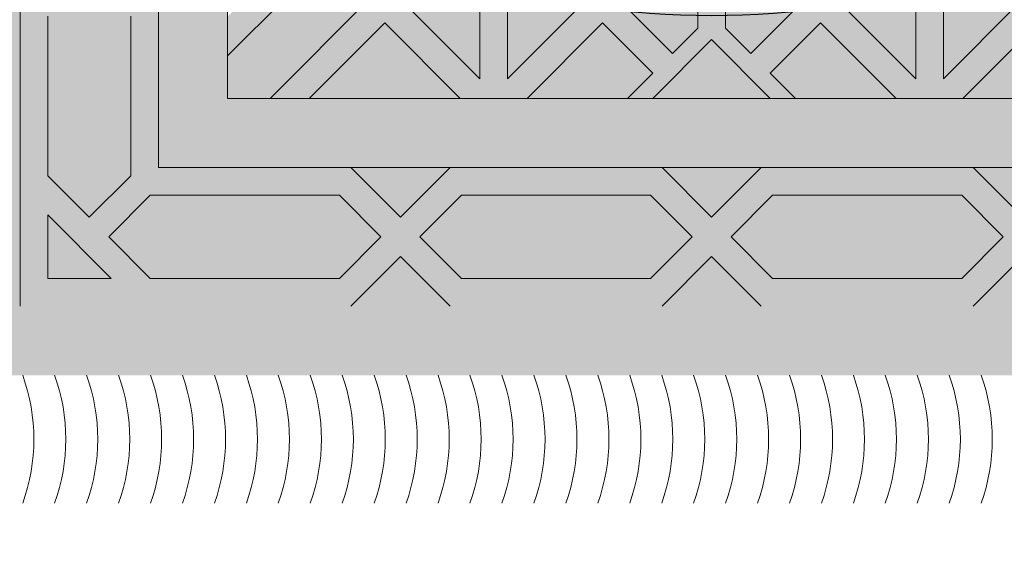
# Model space of a CAD drawing. Units: inches. Extents: x 844 to 2234, y 346 to 1084.
# Tile 69 of 93: x 1997.478 to 2006.557, y 687.628 to 692.525. Entities that reach past the tile are written whole.
import ezdxf

# ---------------------------------------------------------------- set-up
doc = ezdxf.new("R2010")
doc.units = ezdxf.units.IN
doc.header["$MEASUREMENT"] = 0
for name, color, linetype, lineweight in [('A-ANNO-DIMS', 2, 'Continuous', 18), ('furniture', 8, 'Continuous', 18), ('RA-AP-01$0$INT', 35, 'Continuous', 5)]:
    doc.layers.add(name, color=color, linetype=linetype, lineweight=lineweight)
doc.layers.add('RA-AP-01$0$FURN', color=3, linetype='Continuous')
doc.layers.add('RA-AP-01$0$WOOD', color=64, linetype='Continuous')
doc.styles.get("Standard").update_dxf_attribs({"font": 'arial.ttf'})
doc.dimstyles.get("Standard").update_dxf_attribs({"dimtxt": 6, "dimasz": 3, "dimexe": 0.18, "dimexo": 0.0625, "dimgap": 0.09, "dimtad": 0, "dimtih": 1, "dimtoh": 1, "dimdec": 1, "dimzin": 0, "dimdsep": 46, "dimlunit": 3, "dimtxsty": 'Standard', "dimblk": 'ARCHTICK', "dimcen": 0.09, "dimadec": 0, "dimazin": 0, "dimtfac": 1, "dimtdec": 1, "dimtofl": 0, "dimtmove": 0, "dimatfit": 3, "dimfxl": 1, "dimtolj": 1, "dimtzin": 0, "dimarcsym": 0})

# ---------------------------------------------------------------- blocks, each defined once
blk = doc.blocks.new('A$C18D01794')
at = {"layer": 'RA-AP-01$0$INT'}
h = blk.add_hatch(color=256, dxfattribs=at)
h.paths.add_polyline_path([(4.35521, -6.15671), (4.35521, -8.05671), (5.45521, -8.05671), (5.45521, -6.15671)])
h.paths.add_polyline_path([(4.40521, -8.00671), (4.40521, -6.20671), (5.40521, -6.20671), (5.40521, -8.00671)], flags=16)
h = blk.add_hatch(color=256, dxfattribs=at)
h.paths.add_polyline_path([(4.46935, -7.07085), (4.50521, -7.035), (4.50521, -7.10671)])
h.paths.add_polyline_path([(4.45521, -7.085), (4.47692, -7.10671), (4.43349, -7.10671)])
h.paths.add_polyline_path([(4.40521, -7.035), (4.44106, -7.07085), (4.40521, -7.10671)])
h.paths.add_polyline_path([(4.42521, -6.91146), (4.45521, -6.88146), (4.48521, -6.91146), (4.48521, -7.02671), (4.45521, -7.05671), (4.42521, -7.02671)])
h.paths.add_polyline_path([(4.50521, -6.83146), (4.50521, -6.90318), (4.46935, -6.86732)])
h.paths.add_polyline_path([(4.42521, -6.70793), (4.45521, -6.67793), (4.48521, -6.70793), (4.48521, -6.82318), (4.45521, -6.85318), (4.42521, -6.82318)])
h.paths.add_polyline_path([(4.42521, -6.50439), (4.45521, -6.47439), (4.48521, -6.50439), (4.48521, -6.61964), (4.45521, -6.64964), (4.42521, -6.61964)])
h.paths.add_polyline_path([(4.46935, -6.66378), (4.50521, -6.62793), (4.50521, -6.69964)])
h.paths.add_polyline_path([(4.40521, -6.62793), (4.44106, -6.66378), (4.40521, -6.69964)])
h.paths.add_polyline_path([(4.40521, -6.42439), (4.44106, -6.46025), (4.40521, -6.49611)])
h.paths.add_polyline_path([(4.46935, -6.46025), (4.50521, -6.42439), (4.50521, -6.49611)])
h.paths.add_polyline_path([(4.42521, -6.30085), (4.45521, -6.27085), (4.48521, -6.30085), (4.48521, -6.41611), (4.45521, -6.44611), (4.42521, -6.41611)])
h.paths.add_polyline_path([(4.42521, -6.22671), (4.47106, -6.22671), (4.42521, -6.27257)])
h.paths.add_polyline_path([(4.49935, -6.22671), (4.63606, -6.22671), (4.66606, -6.25671), (4.63606, -6.28671), (4.49935, -6.28671), (4.46935, -6.25671)])
h.paths.add_polyline_path([(4.68021, -6.27085), (4.71606, -6.30671), (4.64435, -6.30671)])
h.paths.add_polyline_path([(4.64435, -6.20671), (4.71606, -6.20671), (4.68021, -6.24257)])
h.paths.add_polyline_path([(4.72435, -6.22671), (4.86106, -6.22671), (4.89106, -6.25671), (4.86106, -6.28671), (4.72435, -6.28671), (4.69435, -6.25671)])
h.paths.add_polyline_path([(4.90521, -6.27085), (4.94106, -6.30671), (4.86935, -6.30671)])
h.paths.add_polyline_path([(4.86935, -6.20671), (4.94106, -6.20671), (4.90521, -6.24257)])
h.paths.add_polyline_path([(4.94935, -6.22671), (5.08606, -6.22671), (5.11606, -6.25671), (5.08606, -6.28671), (4.94935, -6.28671), (4.91935, -6.25671)])
h.paths.add_polyline_path([(5.13021, -6.27085), (5.16606, -6.30671), (5.09435, -6.30671)])
h.paths.add_polyline_path([(5.09435, -6.20671), (5.16606, -6.20671), (5.13021, -6.24257)])
h.paths.add_polyline_path([(5.17435, -6.22671), (5.31106, -6.22671), (5.34106, -6.25671), (5.31106, -6.28671), (5.17435, -6.28671), (5.14435, -6.25671)])
h.paths.add_polyline_path([(5.32521, -6.30085), (5.35521, -6.27085), (5.38521, -6.30085), (5.38521, -6.41611), (5.35521, -6.44611), (5.32521, -6.41611)])
h.paths.add_polyline_path([(5.33935, -6.22671), (5.38521, -6.22671), (5.38521, -6.27257)])
h.paths.add_polyline_path([(5.32521, -6.50439), (5.35521, -6.47439), (5.38521, -6.50439), (5.38521, -6.61964), (5.35521, -6.64964), (5.32521, -6.61964)])
h.paths.add_polyline_path([(5.30521, -6.42439), (5.34106, -6.46025), (5.30521, -6.49611)])
h.paths.add_polyline_path([(5.36935, -6.46025), (5.40521, -6.42439), (5.40521, -6.49611)])
h.paths.add_polyline_path([(5.40521, -6.62793), (5.40521, -6.69964), (5.36935, -6.66378)])
h.paths.add_polyline_path([(5.30521, -6.62793), (5.34106, -6.66378), (5.30521, -6.69964)])
h.paths.add_polyline_path([(5.32521, -6.70793), (5.35521, -6.67793), (5.38521, -6.70793), (5.38521, -6.82318), (5.35521, -6.85318), (5.32521, -6.82318)])
h.paths.add_polyline_path([(5.30521, -6.83146), (5.34106, -6.86732), (5.30521, -6.90318)])
h.paths.add_polyline_path([(5.32521, -6.91146), (5.35521, -6.88146), (5.38521, -6.91146), (5.38521, -7.02671), (5.35521, -7.05671), (5.32521, -7.02671)])
h.paths.add_polyline_path([(5.40458, -6.83209, 0.001218), (5.40521, -6.83231), (5.40521, -6.90318), (5.36935, -6.86732)])
h.paths.add_polyline_path([(5.36935, -7.07085), (5.40521, -7.035), (5.40521, -7.10671)])
h.paths.add_polyline_path([(5.35521, -7.085), (5.37692, -7.10671), (5.33349, -7.10671)])
h.paths.add_polyline_path([(5.30521, -7.035), (5.34106, -7.07085), (5.30521, -7.10671)])
h = blk.add_hatch(color=256, dxfattribs=at)
h.paths.add_polyline_path([(4.50521, -6.62793), (4.46935, -6.66378), (4.50521, -6.69964), (4.50521, -6.83146), (4.46935, -6.86732), (4.50521, -6.90318), (4.50521, -7.035), (4.46935, -7.07085), (4.50521, -7.10671), (4.47692, -7.10671), (4.45521, -7.085), (4.43349, -7.10671), (4.40521, -7.10671), (4.44106, -7.07085), (4.40521, -7.035), (4.40521, -6.90318), (4.44106, -6.86732), (4.40521, -6.83146), (4.40521, -6.69964), (4.44106, -6.66378), (4.40521, -6.62793), (4.40521, -6.49611), (4.44106, -6.46025), (4.40521, -6.42439), (4.40521, -6.20671), (4.64435, -6.20671), (4.68021, -6.24257), (4.71606, -6.20671), (4.86935, -6.20671), (4.90521, -6.24257), (4.94106, -6.20671), (5.09435, -6.20671), (5.13021, -6.24257), (5.16606, -6.20671), (5.40521, -6.20671), (5.40521, -6.42439), (5.36935, -6.46025), (5.40521, -6.49611), (5.40521, -6.62793), (5.36935, -6.66378), (5.40521, -6.69964), (5.40521, -6.83146), (5.36935, -6.86732), (5.40521, -6.90318), (5.40521, -7.035), (5.36935, -7.07085), (5.40521, -7.10671), (5.37692, -7.10671), (5.35521, -7.085), (5.33349, -7.10671), (5.30521, -7.10671), (5.34106, -7.07085), (5.30521, -7.035), (5.30521, -6.90318), (5.34106, -6.86732), (5.30521, -6.83146), (5.30521, -6.69964), (5.34106, -6.66378), (5.30521, -6.62793), (5.30521, -6.49611), (5.34106, -6.46025), (5.30521, -6.42439), (5.30521, -6.30671), (5.16606, -6.30671), (5.13021, -6.27085), (5.09435, -6.30671), (4.94106, -6.30671), (4.90521, -6.27085), (4.86935, -6.30671), (4.71606, -6.30671), (4.68021, -6.27085), (4.64435, -6.30671), (4.50521, -6.30671), (4.50521, -6.42439), (4.46935, -6.46025), (4.50521, -6.49611)])
h.paths.add_polyline_path([(4.48521, -6.50439), (4.45521, -6.47439), (4.42521, -6.50439), (4.42521, -6.61964), (4.45521, -6.64964), (4.48521, -6.61964)], flags=16)
h.paths.add_polyline_path([(4.45521, -6.44611), (4.48521, -6.41611), (4.48521, -6.30085), (4.45521, -6.27085), (4.42521, -6.30085), (4.42521, -6.41611)], flags=16)
h.paths.add_polyline_path([(4.45521, -6.67793), (4.42521, -6.70793), (4.42521, -6.82318), (4.45521, -6.85318), (4.48521, -6.82318), (4.48521, -6.70793)], flags=16)
h.paths.add_polyline_path([(4.49935, -6.28671), (4.63606, -6.28671), (4.66606, -6.25671), (4.63606, -6.22671), (4.49935, -6.22671), (4.46935, -6.25671)], flags=16)
h.paths.add_polyline_path([(4.42521, -6.27257), (4.47106, -6.22671), (4.42521, -6.22671)], flags=16)
h.paths.add_polyline_path([(4.45521, -6.88146), (4.42521, -6.91146), (4.42521, -7.02671), (4.45521, -7.05671), (4.48521, -7.02671), (4.48521, -6.91146)], flags=16)
h.paths.add_polyline_path([(4.72435, -6.28671), (4.86106, -6.28671), (4.89106, -6.25671), (4.86106, -6.22671), (4.72435, -6.22671), (4.69435, -6.25671)], flags=16)
h.paths.add_polyline_path([(4.91935, -6.25671), (4.94935, -6.28671), (5.08606, -6.28671), (5.11606, -6.25671), (5.08606, -6.22671), (4.94935, -6.22671)], flags=16)
h.paths.add_polyline_path([(5.14435, -6.25671), (5.17435, -6.28671), (5.31106, -6.28671), (5.34106, -6.25671), (5.31106, -6.22671), (5.17435, -6.22671)], flags=16)
h.paths.add_polyline_path([(5.32521, -6.61964), (5.35521, -6.64964), (5.38521, -6.61964), (5.38521, -6.50439), (5.35521, -6.47439), (5.32521, -6.50439)], flags=16)
h.paths.add_polyline_path([(5.32521, -6.41611), (5.35521, -6.44611), (5.38521, -6.41611), (5.38521, -6.30085), (5.35521, -6.27085), (5.32521, -6.30085)], flags=16)
h.paths.add_polyline_path([(5.32521, -6.70793), (5.32521, -6.82318), (5.35521, -6.85318), (5.38521, -6.82318), (5.38521, -6.70793), (5.35521, -6.67793)], flags=16)
h.paths.add_polyline_path([(5.32521, -6.91146), (5.32521, -7.02671), (5.35521, -7.05671), (5.38521, -7.02671), (5.38521, -6.91146), (5.35521, -6.88146)], flags=16)
h.paths.add_polyline_path([(5.33935, -6.22671), (5.38521, -6.27257), (5.38521, -6.22671)], flags=16)
blk.add_hatch(color=256, dxfattribs=at).paths.add_polyline_path([(4.50521, -6.30671), (5.30521, -6.30671), (5.30521, -7.10671), (5.25521, -7.10671), (5.25521, -6.35671), (4.55521, -6.35671), (4.55521, -7.10671), (4.50521, -7.10671)])
h = blk.add_hatch(color=256, dxfattribs=at)
h.paths.add_polyline_path([(4.58592, -6.35671), (4.55521, -6.35671), (4.55521, -6.38742), (4.8745, -6.70671), (4.90521, -6.676)])
h.paths.add_polyline_path([(5.25521, -6.38742), (5.25521, -6.35671), (5.2245, -6.35671), (4.90521, -6.676), (4.93592, -6.70671)])
h.paths.add_polyline_path([(4.93592, -6.70671), (4.90521, -6.73742), (5.25521, -7.08742), (5.25521, -7.026)])
h.paths.add_polyline_path([(4.55521, -7.026), (4.55521, -7.08742), (4.90521, -6.73742), (4.8745, -6.70671)])
h = blk.add_hatch(color=256, dxfattribs=at)
h.paths.add_polyline_path([(4.58592, -6.35671), (4.6142, -6.35671), (4.66885, -6.41136), (4.72349, -6.35671), (4.77177, -6.35671), (4.82642, -6.41136), (4.86278, -6.375), (4.8445, -6.35671), (4.86278, -6.35671), (4.90521, -6.39914), (4.94763, -6.35671), (4.96592, -6.35671), (4.94763, -6.375), (4.98399, -6.41136), (5.03864, -6.35671), (5.08692, -6.35671), (5.14157, -6.41136), (5.19621, -6.35671), (5.2245, -6.35671), (4.90521, -6.676)])
h.paths.add_polyline_path([(4.89521, -6.63772), (4.89521, -6.52843), (4.84056, -6.58307)], flags=16)
h.paths.add_polyline_path([(4.91521, -6.63772), (4.96985, -6.58307), (4.91521, -6.52843)], flags=16)
h.paths.add_polyline_path([(4.82642, -6.56893), (4.88106, -6.51429), (4.77177, -6.51429)], flags=16)
h.paths.add_polyline_path([(4.98399, -6.56893), (5.03864, -6.51429), (4.92935, -6.51429)], flags=16)
h.paths.add_polyline_path([(4.88106, -6.49429), (4.82642, -6.43964), (4.77177, -6.49429)], flags=16)
h.paths.add_polyline_path([(4.92935, -6.49429), (5.03864, -6.49429), (4.98399, -6.43964)], flags=16)
h.paths.add_polyline_path([(4.89521, -6.48014), (4.89521, -6.40742), (4.87692, -6.38914), (4.84056, -6.4255)], flags=16)
h.paths.add_polyline_path([(4.91521, -6.48014), (4.96985, -6.4255), (4.93349, -6.38914), (4.91521, -6.40742)], flags=16)
h.paths.add_polyline_path([(4.75763, -6.48014), (4.81228, -6.4255), (4.75763, -6.37085)], flags=16)
h.paths.add_polyline_path([(4.73763, -6.48014), (4.73763, -6.37085), (4.68299, -6.4255)], flags=16)
h.paths.add_polyline_path([(5.05278, -6.48014), (5.05278, -6.37085), (4.99814, -6.4255)], flags=16)
h.paths.add_polyline_path([(5.07278, -6.48014), (5.12742, -6.4255), (5.07278, -6.37085)], flags=16)
h.paths.add_polyline_path([(4.93592, -6.70671), (5.25521, -6.38742), (5.25521, -6.41571), (5.20056, -6.47035), (5.25521, -6.525), (5.25521, -6.57328), (5.20056, -6.62793), (5.23692, -6.66429), (5.25521, -6.646), (5.25521, -6.66429), (5.21278, -6.70671), (5.25521, -6.74914), (5.25521, -6.76742), (5.23692, -6.74914), (5.20056, -6.7855), (5.25521, -6.84014), (5.25521, -6.88843), (5.20056, -6.94307), (5.25521, -6.99772), (5.25521, -7.026)])
h.paths.add_polyline_path([(5.04299, -6.7855), (5.09763, -6.84014), (5.09763, -6.73085)], flags=16)
h.paths.add_polyline_path([(5.02885, -6.77136), (5.08349, -6.71671), (4.9742, -6.71671)], flags=16)
h.paths.add_polyline_path([(5.11763, -6.84014), (5.17228, -6.7855), (5.11763, -6.73085)], flags=16)
h.paths.add_polyline_path([(5.08349, -6.69671), (5.02885, -6.64207), (4.9742, -6.69671)], flags=16)
h.paths.add_polyline_path([(5.13177, -6.85429), (5.18642, -6.79964), (5.24106, -6.85429)], flags=17)
h.paths.add_polyline_path([(5.13177, -6.71671), (5.18642, -6.77136), (5.22278, -6.735), (5.2045, -6.71671)], flags=16)
h.paths.add_polyline_path([(5.09763, -6.68257), (5.09763, -6.57328), (5.04299, -6.62793)], flags=16)
h.paths.add_polyline_path([(5.13177, -6.87429), (5.24106, -6.87429), (5.18642, -6.92893)], flags=17)
h.paths.add_polyline_path([(5.13177, -6.69671), (5.2045, -6.69671), (5.22278, -6.67843), (5.18642, -6.64207)], flags=16)
h.paths.add_polyline_path([(5.11763, -6.68257), (5.17228, -6.62793), (5.11763, -6.57328)], flags=16)
h.paths.add_polyline_path([(5.18642, -6.61378), (5.24106, -6.55914), (5.13177, -6.55914)], flags=16)
h.paths.add_polyline_path([(5.13177, -6.53914), (5.24106, -6.53914), (5.18642, -6.48449)], flags=16)
h.paths.add_polyline_path([(5.25521, -7.08742), (5.25521, -7.10671), (4.55521, -7.10671), (4.55521, -7.08742), (4.90521, -6.73742)])
h.paths.add_polyline_path([(4.98399, -6.84449), (4.92935, -6.89914), (5.03864, -6.89914)], flags=16)
h.paths.add_polyline_path([(4.96985, -6.83035), (4.91521, -6.77571), (4.91521, -6.885)], flags=16)
h.paths.add_polyline_path([(4.92935, -6.91914), (4.98399, -6.97378), (5.03864, -6.91914)], flags=16)
h.paths.add_polyline_path([(5.05278, -6.93328), (4.99814, -6.98793), (5.05278, -7.04257)], flags=16)
h.paths.add_polyline_path([(5.07278, -6.93328), (5.07278, -7.04257), (5.12742, -6.98793)], flags=16)
h.paths.add_polyline_path([(4.89521, -6.77571), (4.84056, -6.83035), (4.89521, -6.885)], flags=16)
h.paths.add_polyline_path([(4.91521, -6.93328), (4.91521, -7.006), (4.93349, -7.02429), (4.96985, -6.98793)], flags=16)
h.paths.add_polyline_path([(4.88106, -6.89914), (4.82642, -6.84449), (4.77177, -6.89914)], flags=16)
h.paths.add_polyline_path([(4.89521, -6.93328), (4.84056, -6.98793), (4.87692, -7.02429), (4.89521, -7.006)], flags=16)
h.paths.add_polyline_path([(4.98399, -7.00207), (4.94763, -7.03843), (4.96592, -7.05671), (5.03864, -7.05671)], flags=16)
h.paths.add_polyline_path([(4.88106, -6.91914), (4.77177, -6.91914), (4.82642, -6.97378)], flags=16)
h.paths.add_polyline_path([(4.90521, -7.01429), (4.86278, -7.05671), (4.94763, -7.05671)], flags=16)
h.paths.add_polyline_path([(5.14157, -7.00207), (5.08692, -7.05671), (5.19621, -7.05671)], flags=16)
h.paths.add_polyline_path([(4.82642, -7.00207), (4.77177, -7.05671), (4.8445, -7.05671), (4.86278, -7.03843)], flags=16)
h.paths.add_polyline_path([(4.81228, -6.98793), (4.75763, -6.93328), (4.75763, -7.04257)], flags=16)
h.paths.add_polyline_path([(4.73763, -6.93328), (4.68299, -6.98793), (4.73763, -7.04257)], flags=16)
h.paths.add_polyline_path([(4.72349, -7.05671), (4.66885, -7.00207), (4.6142, -7.05671)], flags=16)
h.paths.add_polyline_path([(4.59763, -6.70671), (4.55521, -6.66429), (4.55521, -6.646), (4.57349, -6.66429), (4.60985, -6.62793), (4.55521, -6.57328), (4.55521, -6.525), (4.60985, -6.47035), (4.55521, -6.41571), (4.55521, -6.38742), (4.8745, -6.70671), (4.55521, -7.026), (4.55521, -6.99772), (4.60985, -6.94307), (4.55521, -6.88843), (4.55521, -6.84014), (4.60985, -6.7855), (4.57349, -6.74914), (4.55521, -6.76742), (4.55521, -6.74914)])
h.paths.add_polyline_path([(4.71278, -6.73085), (4.71278, -6.84014), (4.76742, -6.7855)], flags=16)
h.paths.add_polyline_path([(4.72692, -6.71671), (4.78157, -6.77136), (4.83621, -6.71671)], flags=16)
h.paths.add_polyline_path([(4.69278, -6.73085), (4.63814, -6.7855), (4.69278, -6.84014)], flags=16)
h.paths.add_polyline_path([(4.72692, -6.69671), (4.83621, -6.69671), (4.78157, -6.64207)], flags=16)
h.paths.add_polyline_path([(4.67864, -6.71671), (4.60592, -6.71671), (4.58763, -6.735), (4.62399, -6.77136)], flags=16)
h.paths.add_polyline_path([(4.71278, -6.68257), (4.76742, -6.62793), (4.71278, -6.57328)], flags=16)
h.paths.add_polyline_path([(4.67864, -6.69671), (4.62399, -6.64207), (4.58763, -6.67843), (4.60592, -6.69671)], flags=16)
h.paths.add_polyline_path([(4.69278, -6.68257), (4.69278, -6.57328), (4.63814, -6.62793)], flags=16)
h.paths.add_polyline_path([(4.62399, -6.79964), (4.67864, -6.85429), (4.56935, -6.85429)], flags=17)
h.paths.add_polyline_path([(4.62399, -6.61378), (4.67864, -6.55914), (4.56935, -6.55914)], flags=16)
h.paths.add_polyline_path([(4.67864, -6.87429), (4.62399, -6.92893), (4.56935, -6.87429)], flags=17)
h.paths.add_polyline_path([(4.67864, -6.53914), (4.62399, -6.48449), (4.56935, -6.53914)], flags=16)
h = blk.add_hatch(color=256, dxfattribs=at)
h.paths.add_polyline_path([(4.96985, -6.58307), (4.91521, -6.63772), (4.91521, -6.52843)])
h.paths.add_polyline_path([(4.89521, -6.63772), (4.84056, -6.58307), (4.89521, -6.52843)])
h.paths.add_polyline_path([(4.82642, -6.56893), (4.77177, -6.51429), (4.88106, -6.51429)])
h.paths.add_polyline_path([(4.88106, -6.49429), (4.77177, -6.49429), (4.82642, -6.43964)])
h.paths.add_polyline_path([(4.89521, -6.48014), (4.84056, -6.4255), (4.87692, -6.38914), (4.89521, -6.40742)])
h.paths.add_polyline_path([(4.86278, -6.375), (4.82642, -6.41136), (4.77177, -6.35671), (4.8445, -6.35671)])
h.paths.add_polyline_path([(4.81228, -6.4255), (4.75763, -6.48014), (4.75763, -6.37085)])
h.paths.add_polyline_path([(4.73763, -6.48014), (4.68299, -6.4255), (4.73763, -6.37085)])
h.paths.add_polyline_path([(4.66885, -6.41136), (4.6142, -6.35671), (4.72349, -6.35671)])
h.paths.add_polyline_path([(4.90521, -6.39914), (4.86278, -6.35671), (4.94763, -6.35671)])
h.paths.add_polyline_path([(4.91521, -6.48014), (4.91521, -6.40742), (4.93349, -6.38914), (4.96985, -6.4255)])
h.paths.add_polyline_path([(5.03864, -6.49429), (4.92935, -6.49429), (4.98399, -6.43964)])
h.paths.add_polyline_path([(4.98399, -6.56893), (4.92935, -6.51429), (5.03864, -6.51429)])
h.paths.add_polyline_path([(5.05278, -6.48014), (4.99814, -6.4255), (5.05278, -6.37085)])
h.paths.add_polyline_path([(4.98399, -6.41136), (4.94763, -6.375), (4.96592, -6.35671), (5.03864, -6.35671)])
h.paths.add_polyline_path([(5.12742, -6.4255), (5.07278, -6.48014), (5.07278, -6.37085)])
h.paths.add_polyline_path([(5.14157, -6.41136), (5.08692, -6.35671), (5.19621, -6.35671)])
for p, q in [((4.71606, -6.20671), (4.68021, -6.24257)), ((4.86935, -6.20671), (4.90521, -6.24257)), ((4.94106, -6.20671), (4.90521, -6.24257)), ((5.09435, -6.20671), (5.13021, -6.24257)), ((5.16606, -6.20671), (5.13021, -6.24257)), ((4.72435, -6.22671), (4.69435, -6.25671)), ((4.86106, -6.22671), (4.72435, -6.22671)), ((4.86106, -6.22671), (4.89106, -6.25671)), ((4.94935, -6.22671), (4.91935, -6.25671)), ((4.94935, -6.22671), (5.08606, -6.22671)), ((5.08606, -6.22671), (5.11606, -6.25671)), ((5.17435, -6.22671), (5.14435, -6.25671)), ((5.17435, -6.22671), (5.31106, -6.22671)), ((5.31106, -6.22671), (5.34106, -6.25671)), ((5.33935, -6.22671), (5.38521, -6.27257)), ((5.33935, -6.22671), (5.38521, -6.22671)), ((5.38521, -6.27257), (5.38521, -6.22671)), ((4.72435, -6.28671), (4.69435, -6.25671)), ((4.86106, -6.28671), (4.89106, -6.25671)), ((4.94935, -6.28671), (4.91935, -6.25671)), ((5.08606, -6.28671), (5.11606, -6.25671)), ((5.17435, -6.28671), (5.14435, -6.25671)), ((5.31106, -6.28671), (5.34106, -6.25671)), ((4.71606, -6.30671), (4.68021, -6.27085)), ((4.86935, -6.30671), (4.90521, -6.27085)), ((4.94106, -6.30671), (4.90521, -6.27085)), ((5.09435, -6.30671), (5.13021, -6.27085)), ((5.16606, -6.30671), (5.13021, -6.27085)), ((5.32521, -6.30085), (5.35521, -6.27085)), ((5.38521, -6.30085), (5.35521, -6.27085)), ((4.86106, -6.28671), (4.72435, -6.28671)), ((4.94935, -6.28671), (5.08606, -6.28671)), ((5.17435, -6.28671), (5.31106, -6.28671)), ((5.26721, -6.30671), (4.54321, -6.30671)), ((5.26721, -6.30671), (4.54321, -6.30671)), ((5.32521, -6.30085), (5.32521, -6.41611)), ((5.38521, -6.41611), (5.38521, -6.30085)), ((4.55521, -6.35671), (5.25521, -6.35671)), ((4.72349, -6.35671), (4.66885, -6.41136)), ((4.77177, -6.35671), (4.82642, -6.41136)), ((4.8445, -6.35671), (4.77177, -6.35671)), ((4.8445, -6.35671), (4.86278, -6.375)), ((4.94763, -6.35671), (4.86278, -6.35671)), ((4.90521, -6.39914), (4.86278, -6.35671)), ((4.90521, -6.39914), (4.94763, -6.35671)), ((4.90521, -6.676), (5.2245, -6.35671)), ((4.96592, -6.35671), (4.94763, -6.375)), ((4.94763, -6.375), (4.96592, -6.35671)), ((4.96592, -6.35671), (5.03864, -6.35671)), ((5.03864, -6.35671), (4.98399, -6.41136)), ((5.08692, -6.35671), (5.14157, -6.41136)), ((5.19621, -6.35671), (5.14157, -6.41136)), ((5.25521, -7.10671), (5.25521, -6.35671)), ((4.73763, -6.37085), (4.68299, -6.4255)), ((4.73763, -6.48014), (4.73763, -6.37085)), ((4.75763, -6.48014), (4.75763, -6.37085)), ((4.75763, -6.37085), (4.81228, -6.4255)), ((5.05278, -6.37085), (4.99814, -6.4255)), ((5.05278, -6.48014), (5.05278, -6.37085)), ((5.07278, -6.48014), (5.07278, -6.37085)), ((5.07278, -6.37085), (5.12742, -6.4255)), ((4.82642, -6.41136), (4.86278, -6.375)), ((4.98399, -6.41136), (4.94763, -6.375)), ((4.84056, -6.4255), (4.87692, -6.38914)), ((4.89521, -6.40742), (4.87692, -6.38914)), ((4.91521, -6.40742), (4.93349, -6.38914)), ((4.96985, -6.4255), (4.93349, -6.38914)), ((4.93592, -6.70671), (5.25521, -6.38742)), ((4.89521, -6.40742), (4.89521, -6.48014)), ((4.91521, -6.40742), (4.91521, -6.48014))]:
    blk.add_line(p, q, dxfattribs=at)
for points in [[(5.40521, -7.10671), (5.40521, -6.20671)], [(5.30521, -7.10671), (5.30521, -6.30671), (4.50521, -6.30671), (4.50521, -7.10671)]]:
    blk.add_lwpolyline(points, dxfattribs=at)
for centre in [(4.83866, -6.11051), (4.86176, -6.11051), (4.88486, -6.11051), (4.90796, -6.11051), (4.93106, -6.11051), (4.95416, -6.11051), (4.97726, -6.11051), (5.00036, -6.11051), (5.02346, -6.11051), (5.04656, -6.11051), (5.06966, -6.11051), (5.09276, -6.11051), (5.11586, -6.11051), (5.13896, -6.11051), (5.16206, -6.11051), (5.18516, -6.11051), (5.20826, -6.11051), (5.23136, -6.11051), (5.25446, -6.11051), (5.27756, -6.11051), (5.30066, -6.11051), (5.32376, -6.11051), (5.34686, -6.11051), (5.36996, -6.11051), (5.39306, -6.11051), (5.41616, -6.11051), (5.43926, -6.11051), (5.46236, -6.11051), (5.48546, -6.11051), (5.50856, -6.11051), (5.53166, -6.11051)]:
    blk.add_arc(centre, 0.13641, 160.20384, 199.79616, dxfattribs=at)
blk = doc.blocks.new('A$C32926AE1')
at = {"layer": 'RA-AP-01$0$WOOD'}
blk.add_arc((4.90477, 4.06706), 0.4604, 252.0684, 287.9316, dxfattribs=at)
blk = doc.blocks.new('A$C5D2F253E')
at = {"layer": 'RA-AP-01$0$FURN', "xscale": -0.7999999999883585, "yscale": 0.7999999999883585, "zscale": 0.8, "rotation": 90}
blk.add_blockref('A$C18D01794', (-5.68776, 4.75792), dxfattribs=at)
at = {"layer": 'RA-AP-01$0$WOOD', "rotation": 270}
blk.add_blockref('A$C32926AE1', (-4.16134, 5.73853), dxfattribs=at)
blk = doc.blocks.new('_ArchTick')
at = {"color": 0, "linetype": 'ByBlock', "const_width": 0.15}
blk.add_lwpolyline([(-0.5, -0.5), (0.5, 0.5)], dxfattribs=at)
blk = doc.blocks.new('*D121')
at = {"layer": 'A-ANNO-DIMS', "color": 0, "lineweight": -2, "transparency": 16777216}
for p, q in [((2030.272, 734.2626), (2040.2453, 734.2626)), ((2040.0653, 734.2626), (2040.0653, 704.6044)), ((2040.0653, 668.5574), (2040.0653, 698.2156)), ((2030.272, 668.5574), (2040.2453, 668.5574))]:
    blk.add_line(p, q, dxfattribs=at)
at = {"layer": 'Defpoints', "color": 0, "transparency": 16777216}
for p in [(2030.2095, 734.2626), (2040.0653, 734.2626), (2030.2095, 668.5574)]:
    blk.add_point(p, dxfattribs=at)
at = {"layer": 'A-ANNO-DIMS', "color": 0, "lineweight": -2, "transparency": 16777216, "xscale": 3, "yscale": 3, "zscale": 3}
for p, rotation in [((2040.0653, 734.2626), 90), ((2040.0653, 668.5574), 270)]:
    blk.add_blockref('_ArchTick', p, dxfattribs=dict(at, rotation=rotation))
at = {"layer": 'A-ANNO-DIMS', "color": 0, "transparency": 16777216, "insert": (2040.0653, 701.41), "char_height": 6, "attachment_point": 5}
blk.add_mtext('\\A1;LOUNGE SET 5\'-5 1/2" TYP.', dxfattribs=at)

msp = doc.modelspace()

# ---------------------------------------------------------------- block references
at = {"layer": 'furniture', "xscale": -15.94108302203742, "yscale": 15.94108302203742, "zscale": 15.94108302203742, "rotation": 270}
msp.add_blockref('A$C5D2F253E', (1990.5673, 701.4029), dxfattribs=at)

# ---------------------------------------------------------------- dimensions: what is measured, and where the dimension line sits
at = {"layer": 'A-ANNO-DIMS'}
dim = msp.add_linear_dim(base=(2040.0653, 734.2626), p1=(2030.2095, 668.5574), p2=(2030.2095, 734.2626), angle=90, text='LOUNGE SET <> TYP.', dimstyle='Standard', override={"dimdec": 1, "dimlfac": 1, "dimrnd": 0, "dimzin": 1, "dimdsep": 46, "dimlunit": 4, "dimfrac": 2}, dxfattribs=at)
dim.commit()
dim.dimension.update_dxf_attribs({"geometry": '*D121', "text_midpoint": (2040.0653, 701.41)})

doc.saveas('drawing.dxf')
